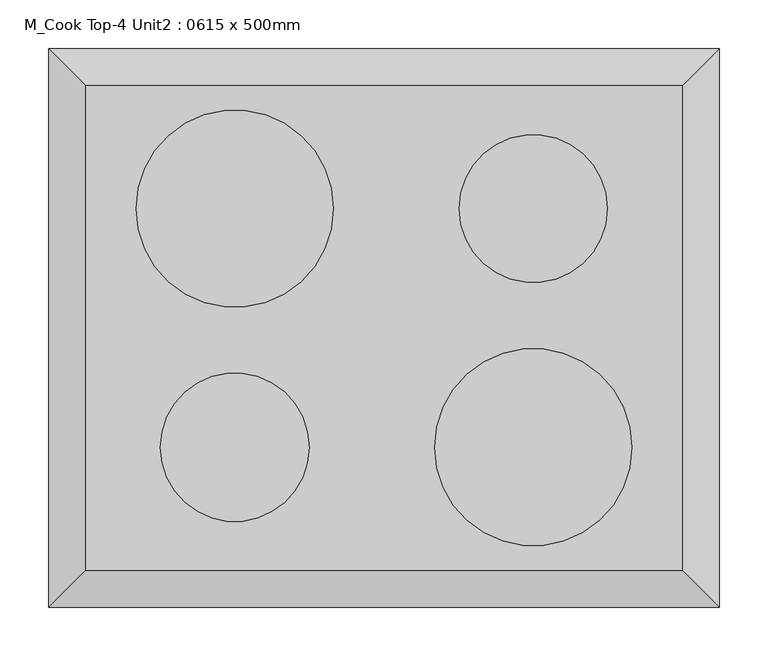
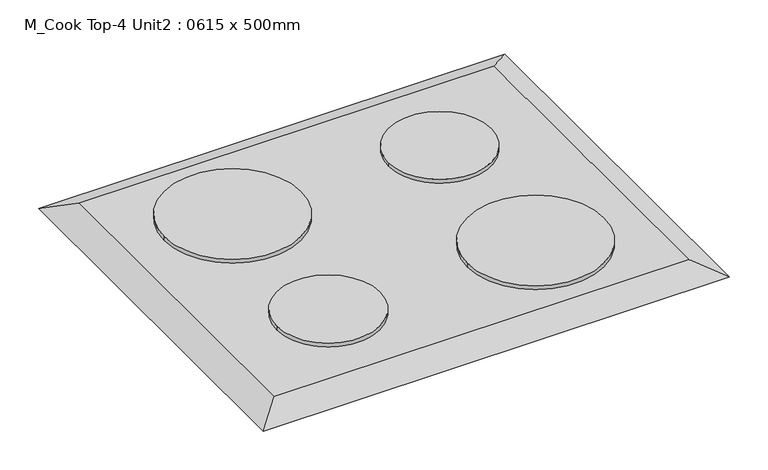
"""IFC4 building model written with IfcOpenShell, lengths in millimetres: proxy geometry, M_Cook Top-4 Unit2 : 0615 x 500mm."""

from ifc_helpers import new_model, si_unit, point, frame, frame_2d, origin, place, context, project, spatial, circle_curve, trimmed, segment, composite_curve, outline, extrude, faceted_brep, source, transform, mapped, element, save


def m_cook_top_4_unit2_0615_x_500mm_c91639ce(model_context):
    return source(origin(), model_context, "Body", "SolidModel", [
        faceted_brep([(307.5, -250.0, 918.0), (307.5, 250.0, 918.0), (-307.5, 250.0, 918.0), (-307.5, -250.0, 918.0), (345.6, -288.1, 900.0), (-345.6, -288.1, 900.0), (-345.6, 288.1, 900.0), (345.6, 288.1, 900.0)], [[[0, 1, 2, 3]], [[4, 5, 6, 7]], [[4, 0, 3, 5]], [[5, 3, 2, 6]], [[6, 2, 1, 7]], [[7, 1, 0, 4]]]),
        extrude(outline(composite_curve([segment(trimmed(circle_curve(frame_2d((153.75, 123.0)), 76.2), [point((77.55, 123.0))], [point((229.95, 123.0))], False, "CARTESIAN"), True, "CONTINUOUS"), segment(trimmed(circle_curve(frame_2d((153.75, 123.0)), 76.2), [point((229.95, 123.0))], [point((77.55, 123.0))], False, "CARTESIAN"), True, "CONTINUOUS")], self_intersect=False)), frame((0.0, 0.0, 918.0), z_axis=(0.0, 0.0, 1.0), x_axis=(1.0, 0.0, 0.0)), (0.0, 0.0, 1.0), 6.35),
        extrude(outline(composite_curve([segment(trimmed(circle_curve(frame_2d((153.75, -123.0)), 101.6), [point((52.15, -123.0))], [point((255.35, -123.0))], False, "CARTESIAN"), True, "CONTINUOUS"), segment(trimmed(circle_curve(frame_2d((153.75, -123.0)), 101.6), [point((255.35, -123.0))], [point((52.15, -123.0))], False, "CARTESIAN"), True, "CONTINUOUS")], self_intersect=False)), frame((0.0, 0.0, 918.0), z_axis=(0.0, 0.0, 1.0), x_axis=(1.0, 0.0, 0.0)), (0.0, 0.0, 1.0), 6.35),
        extrude(outline(composite_curve([segment(trimmed(circle_curve(frame_2d((-153.75, -123.0)), 76.59), [point((-230.34, -123.0))], [point((-77.16, -123.0))], False, "CARTESIAN"), True, "CONTINUOUS"), segment(trimmed(circle_curve(frame_2d((-153.75, -123.0)), 76.59), [point((-77.16, -123.0))], [point((-230.34, -123.0))], False, "CARTESIAN"), True, "CONTINUOUS")], self_intersect=False)), frame((0.0, 0.0, 918.0), z_axis=(0.0, 0.0, 1.0), x_axis=(1.0, 0.0, 0.0)), (0.0, 0.0, 1.0), 6.35),
        extrude(outline(composite_curve([segment(trimmed(circle_curve(frame_2d((-153.75, 123.0)), 101.6), [point((-52.15, 123.0))], [point((-255.35, 123.0))], False, "CARTESIAN"), True, "CONTINUOUS"), segment(trimmed(circle_curve(frame_2d((-153.75, 123.0)), 101.6), [point((-255.35, 123.0))], [point((-52.15, 123.0))], False, "CARTESIAN"), True, "CONTINUOUS")], self_intersect=False)), frame((0.0, 0.0, 918.0), z_axis=(0.0, 0.0, 1.0), x_axis=(1.0, 0.0, 0.0)), (0.0, 0.0, 1.0), 6.35),
    ])


if __name__ == "__main__":
    model = new_model("IFC4")
    model_context = context("Model", 3, world=origin())
    ifc_project = project(units=[si_unit("LENGTHUNIT", "METRE", prefix="MILLI")], contexts=[model_context])
    site = spatial("IfcSite", under=ifc_project)
    building = spatial("IfcBuilding", under=site)
    placement = place(None, origin())
    m_cook_top_4_unit2_0615_x_500mm_shape = m_cook_top_4_unit2_0615_x_500mm_c91639ce(model_context)
    element("IfcBuildingElementProxy", 1, Name="M_Cook Top-4 Unit2 : 0615 x 500mm", ObjectType="M_Cook Top-4 Unit2 : 0615 x 500mm", at=placement, inside=building, context=model_context, shape_type="MappedRepresentation", body=[
        mapped(m_cook_top_4_unit2_0615_x_500mm_shape, transform((0.0, 0.0, 0.0), x_axis=(1.0, 0.0, 0.0), y_axis=(0.0, 1.0, 0.0), z_axis=(0.0, 0.0, 1.0))),
    ])
    save(model, "model.ifc")

# Revit data of these elements
# Type "M_Cook Top-4 Unit2 : 0615 x 500mm"
#   Depth = 1.64042 ft
#   Width = 2.017717 ft
#   Burner Material = Steel, Chrome Plated
#   Cooktop Material = Steel, Polished
#   Default Elevation = 0
#   Assembly Code = ""
# Element 1 (IfcBuildingElementProxy, "M_Cook Top-4 Unit2 : 0615 x 500mm")
#   Materials on its faces: "Steel, Polished", "Steel, Chrome Plated"
# Materials
#   "Steel, Chrome Plated": class "Metal", colour RGB 17 17 17, transparency 0, Description = "Chromiuim plated steel", Cost = 0
#   "Steel, Polished": class "Metal", colour RGB 57 57 57, transparency 0, Description = "Polished steel", Cost = 0
